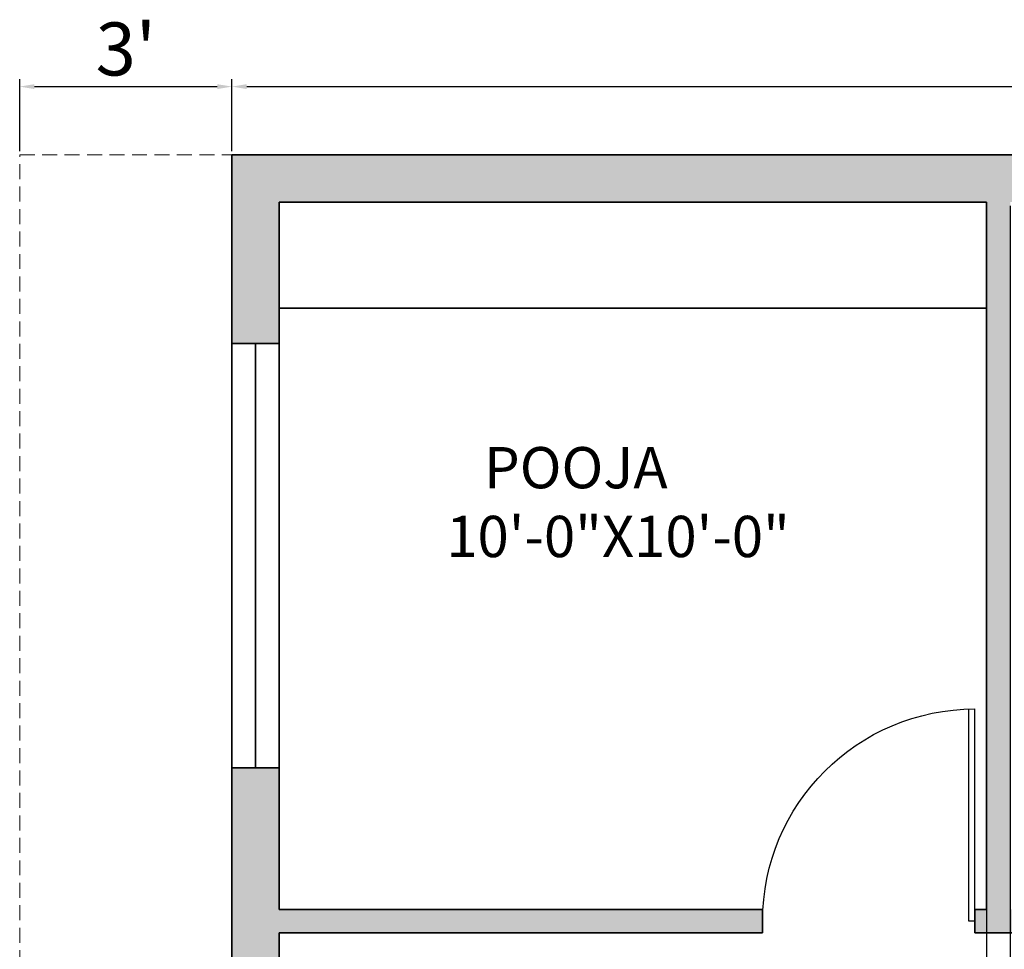
# Model space of a CAD drawing. Units: inches. Extents: x 1566 to 2546, y 1087 to 2705.
# Tile 10 of 27: x 1606 to 1773, y 1643 to 1801. Entities that reach past the tile are written whole.
import ezdxf

# ---------------------------------------------------------------- set-up
doc = ezdxf.new("R2010")
doc.units = ezdxf.units.IN
doc.linetypes.add('DASHED', pattern=[19.05, 12.7, -6.35])
for name, color, linetype, lineweight in [('A-ANNO-DIMS', 2, 'Continuous', 18), ('A-AREA-IDEN', 7, 'Continuous', 18), ('A-DOOR', 4, 'Continuous', 25), ('A-FLOR-OVHD', 8, 'DASHED', 18), ('A-WALL', 7, 'Continuous', 35), ('A-WALL-PATT', 8, 'Continuous', 13)]:
    doc.layers.add(name, color=color, linetype=linetype, lineweight=lineweight)
doc.styles.get("Standard").update_dxf_attribs({"font": 'arial.ttf'})
doc.dimstyles.new('ISO-25', dxfattribs={"dimtxt": 2.5, "dimasz": 2.5, "dimexe": 1.25, "dimexo": 0.625, "dimtad": 1, "dimtxsty": 'Standard', "dimcen": 2.5, "dimadec": 0, "dimazin": 0, "dimtfac": 1, "dimtmove": 0, "dimatfit": 3, "dimfxl": 1, "dimarcsym": 0})

# ---------------------------------------------------------------- blocks, each defined once
blk = doc.blocks.new('d1')
for p, q in [((3297.32, 1596.93), (3297.32, 1632.93)), ((3298.32, 1596.93), (3298.32, 1632.93)), ((3297.32, 1596.93), (3298.32, 1596.93))]:
    blk.add_line(p, q)
at = {"ltscale": 0.3}
blk.add_arc((3297.32, 1596.93), 36, 0, 90, dxfattribs=at)
blk = doc.blocks.new('*D9')
at = {"layer": 'A-ANNO-DIMS', "color": 0, "lineweight": -2, "transparency": 16777216}
for p, q in [((1641.53, 1778.82), (1641.53, 1791.04)), ((2001.53, 1778.82), (2001.53, 1791.04)), ((1644.03, 1789.79), (1999.03, 1789.79))]:
    blk.add_line(p, q, dxfattribs=at)
at = {"layer": 'A-ANNO-DIMS', "color": 0, "transparency": 16777216}
for points in [[(1644.03, 1790.2), (1644.03, 1789.37), (1641.53, 1789.79)], [(1999.03, 1790.2), (1999.03, 1789.37), (2001.53, 1789.79)]]:
    blk.add_solid(points, dxfattribs=at)
at = {"layer": 'Defpoints', "color": 0, "transparency": 16777216}
for p in [(2001.53, 1789.79), (1641.53, 1778.2), (2001.53, 1778.2)]:
    blk.add_point(p, dxfattribs=at)
at = {"layer": 'A-ANNO-DIMS', "color": 0, "transparency": 16777216, "insert": (1821.53, 1795.01), "char_height": 9, "attachment_point": 5}
blk.add_mtext("30'", dxfattribs=at)
blk = doc.blocks.new('*D10')
at = {"layer": 'A-ANNO-DIMS', "color": 0, "lineweight": -2, "transparency": 16777216}
for p, q in [((1605.53, 1778.82), (1605.53, 1791.04)), ((1641.53, 1778.82), (1641.53, 1791.04)), ((1608.03, 1789.79), (1639.03, 1789.79))]:
    blk.add_line(p, q, dxfattribs=at)
at = {"layer": 'A-ANNO-DIMS', "color": 0, "transparency": 16777216}
for points in [[(1608.03, 1790.2), (1608.03, 1789.37), (1605.53, 1789.79)], [(1639.03, 1790.2), (1639.03, 1789.37), (1641.53, 1789.79)]]:
    blk.add_solid(points, dxfattribs=at)
at = {"layer": 'Defpoints', "color": 0, "transparency": 16777216}
for p in [(1641.53, 1789.79), (1605.53, 1778.2), (1641.53, 1778.2)]:
    blk.add_point(p, dxfattribs=at)
at = {"layer": 'A-ANNO-DIMS', "color": 0, "transparency": 16777216, "insert": (1623.53, 1795.01), "char_height": 9, "attachment_point": 5}
blk.add_mtext("3'", dxfattribs=at)
blk = doc.blocks.new('*D110')
at = {"layer": 'A-ANNO-DIMS', "color": 0, "lineweight": -2, "transparency": 16777216}
for p, q in [((1769.53, 1769.57), (1769.53, 1087.35)), ((1773.53, 1769.57), (1773.53, 1087.35)), ((1767.03, 1088.6), (1764.53, 1088.6)), ((1769.53, 1088.6), (1773.53, 1088.6)), ((1776.03, 1088.6), (1786.43, 1088.6))]:
    blk.add_line(p, q, dxfattribs=at)
at = {"layer": 'A-ANNO-DIMS', "color": 0, "transparency": 16777216}
for points in [[(1767.03, 1089.01), (1767.03, 1088.18), (1769.53, 1088.6)], [(1776.03, 1089.01), (1776.03, 1088.18), (1773.53, 1088.6)]]:
    blk.add_solid(points, dxfattribs=at)
at = {"layer": 'Defpoints', "color": 0, "transparency": 16777216}
for p in [(1769.53, 1770.2), (1773.53, 1770.2), (1773.53, 1088.6)]:
    blk.add_point(p, dxfattribs=at)
at = {"layer": 'A-ANNO-DIMS', "color": 0, "transparency": 16777216, "insert": (1782.48, 1090.5), "char_height": 2.5, "attachment_point": 5}
blk.add_mtext('0\'-4"', dxfattribs=at)

msp = doc.modelspace()

# ---------------------------------------------------------------- hatches: boundary and pattern name
at = {"layer": 'A-WALL-PATT'}
h = msp.add_hatch(color=256, dxfattribs=at)
h.dxf.hatch_style = 1
h.paths.add_polyline_path([(2001.53, 1778.2), (1641.53, 1778.2), (1641.53, 1746.2), (1649.53, 1746.2), (1649.53, 1770.2), (1769.53, 1770.2), (1769.53, 1650.2), (1767.53, 1650.2), (1767.53, 1648.2), (1767.53, 1646.2), (1819.53, 1646.2), (1819.53, 1650.2), (1773.53, 1650.2), (1773.53, 1770.2), (1941.53, 1770.2), (1941.53, 1756.2), (1945.53, 1756.2), (1945.53, 1770.2), (1993.53, 1770.2), (1993.53, 1650.2), (1945.53, 1650.2), (1945.53, 1652.2), (1943.53, 1652.2), (1941.53, 1652.2), (1941.53, 1650.2), (1867.53, 1650.2), (1867.53, 1642.2), (1871.53, 1642.2), (1871.53, 1646.2), (1993.53, 1646.2), (1993.53, 1526.2), (1871.53, 1526.2), (1871.53, 1606.2), (1867.53, 1606.2), (1867.53, 1522.2), (1993.53, 1522.2), (1993.53, 1387.2), (1959.53, 1387.2), (1959.53, 1397.2), (1955.53, 1397.2), (1955.53, 1387.2), (1903.53, 1387.2), (1903.53, 1383.2), (1993.53, 1383.2), (1993.53, 1364.3), (1993.53, 1211.2), (1939.53, 1211.2), (1939.53, 1203.2), (1993.53, 1203.2), (1993.53, 1154.2), (2001.53, 1154.2)])
h.paths.add_polyline_path([(1649.53, 1646.2), (1731.53, 1646.2), (1731.53, 1650.2), (1649.53, 1650.2), (1649.53, 1674.2), (1641.53, 1674.2), (1641.53, 1622.2), (1649.53, 1622.2)], flags=17)
h.paths.add_polyline_path([(1649.53, 1550.2), (1641.53, 1550.2), (1641.53, 1510.2), (1649.53, 1510.2), (1649.53, 1522.2), (1731.53, 1522.2), (1731.53, 1500.2), (1735.53, 1500.2), (1735.53, 1522.2), (1767.53, 1522.2), (1767.53, 1500.2), (1771.53, 1500.2), (1771.53, 1526.2), (1649.53, 1526.2)], flags=17)
h.paths.add_polyline_path([(1649.53, 1464.2), (1735.53, 1464.2), (1735.53, 1470.2), (1731.53, 1470.2), (1731.53, 1468.2), (1649.53, 1468.2), (1649.53, 1480.2), (1641.53, 1480.2), (1641.53, 1419.2), (1649.53, 1419.2)], flags=17)
h.paths.add_polyline_path([(1649.53, 1323.2), (1641.53, 1323.2), (1641.53, 1270.2), (1667.53, 1270.2), (1667.53, 1278.2), (1649.53, 1278.2)], flags=17)
h.paths.add_polyline_path([(1763.53, 1278.2), (1727.53, 1278.2), (1727.53, 1270.2), (1763.53, 1270.2)], flags=17)
h.paths.add_polyline_path([(1823.53, 1383.2), (1827.53, 1383.2), (1827.53, 1385.2), (1827.53, 1387.2), (1819.53, 1387.2), (1819.53, 1324.21), (1819.53, 1278.2), (1811.53, 1278.2), (1811.53, 1274.2), (1811.53, 1270.2), (1819.53, 1270.2), (1819.53, 1203.2), (1877.53, 1203.2), (1877.53, 1211.2), (1823.53, 1211.2)], flags=17)

# ---------------------------------------------------------------- linework, layer by layer
at = {"layer": 'A-FLOR-OVHD', "ltscale": 0.2}
for p, q in [((1605.53, 1130.2), (1605.53, 1778.2)), ((1605.53, 1778.2), (1641.53, 1778.2))]:
    msp.add_line(p, q, dxfattribs=at)
at = {"layer": 'A-WALL'}
for p, q in [((1641.53, 1778.2), (2001.53, 1778.2)), ((1641.53, 1154.2), (1641.53, 1778.2)), ((1649.53, 1770.2), (1769.53, 1770.2)), ((1649.53, 1650.2), (1649.53, 1770.2)), ((1769.53, 1650.2), (1769.53, 1770.2)), ((1649.53, 1752.2), (1769.53, 1752.2)), ((1641.53, 1746.2), (1649.53, 1746.2)), ((1645.53, 1746.2), (1645.53, 1674.2)), ((1649.53, 1674.2), (1641.53, 1674.2)), ((1649.53, 1650.2), (1731.53, 1650.2)), ((1731.53, 1646.2), (1731.53, 1650.2)), ((1767.53, 1646.2), (1767.53, 1650.2)), ((1767.53, 1650.2), (1769.53, 1650.2)), ((1649.53, 1646.2), (1731.53, 1646.2)), ((1649.53, 1526.2), (1649.53, 1646.2)), ((1767.53, 1646.2), (1819.53, 1646.2))]:
    msp.add_line(p, q, dxfattribs=at)

# ---------------------------------------------------------------- block references
at = {"layer": 'A-DOOR', "xscale": -1}
msp.add_blockref('d1', (5064.85, 51.27), dxfattribs=at)

# ---------------------------------------------------------------- texts
at = {"layer": 'A-AREA-IDEN', "insert": (1677.88, 1728.64), "char_height": 7, "attachment_point": 1}
msp.add_mtext_dynamic_manual_height_columns('   POOJA\\P10\'-0"X10\'-0"', width=111.7553, gutter_width=12.5, heights=[0], dxfattribs=at)

# ---------------------------------------------------------------- dimensions: what is measured, and where the dimension line sits
at = {"layer": 'A-ANNO-DIMS'}
for base, p1, p2, override, picture, middle in [((1641.53, 1789.79), (1605.53, 1778.2), (1641.53, 1778.2), {"dimtxt": 9, "dimdec": 1, "dimlunit": 3, "dimclrd": 0, "dimclre": 0, "dimclrt": 0, "dimtdec": 1}, '*D10', (1623.53, 1795.01)), ((2001.53, 1789.79), (1641.53, 1778.2), (2001.53, 1778.2), {"dimtxt": 9, "dimdec": 1, "dimlunit": 3, "dimclrd": 0, "dimclre": 0, "dimclrt": 0, "dimtdec": 1}, '*D9', (1821.53, 1795.01)), ((1773.53, 1088.6), (1769.53, 1770.2), (1773.53, 1770.2), {"dimdec": 1, "dimlfac": 1, "dimrnd": 0, "dimzin": 1, "dimdsep": 46, "dimlunit": 4, "dimfrac": 2}, '*D110', (1782.48, 1090.5))]:
    dim = msp.add_linear_dim(base=base, p1=p1, p2=p2, dimstyle='ISO-25', override=override, dxfattribs=at)
    dim.commit()
    dim.dimension.update_dxf_attribs({"geometry": picture, "text_midpoint": middle})

doc.saveas('drawing.dxf')
